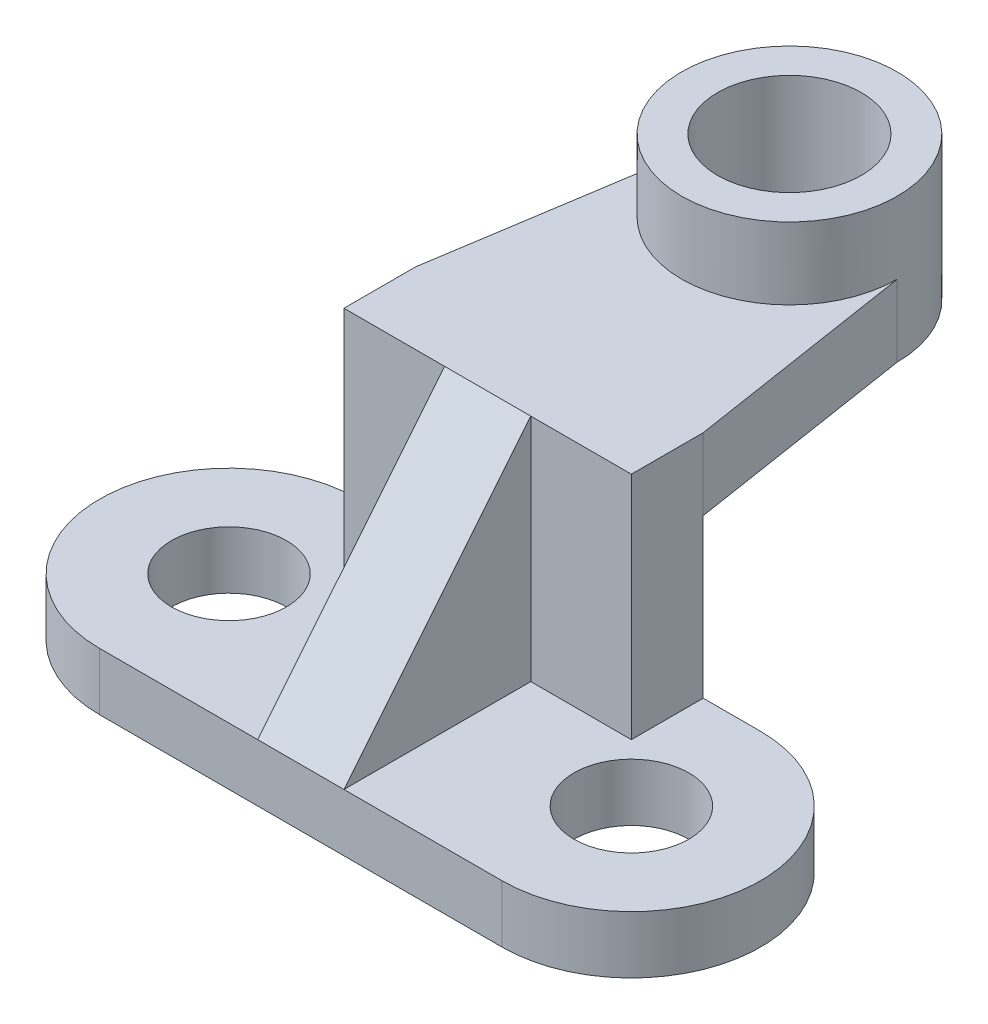
ISO-10303-21;
HEADER;
FILE_DESCRIPTION(('STEP AP214'),'2;1');
FILE_NAME('part.step','',(''),(''),'','','');
FILE_SCHEMA(('AUTOMOTIVE_DESIGN { 1 0 10303 214 1 1 1 1 }'));
ENDSEC;
DATA;
#1=APPLICATION_CONTEXT('core data for automotive mechanical design processes');
#2=APPLICATION_PROTOCOL_DEFINITION('international standard','automotive_design',2000,#1);
#3=PRODUCT_CONTEXT('',#1,'mechanical');
#4=PRODUCT('Part','Part','',(#3));
#5=PRODUCT_RELATED_PRODUCT_CATEGORY('part','',(#4));
#6=PRODUCT_DEFINITION_FORMATION('','',#4);
#7=PRODUCT_DEFINITION_CONTEXT('part definition',#1,'design');
#8=PRODUCT_DEFINITION('design','',#6,#7);
#9=PRODUCT_DEFINITION_SHAPE('','',#8);
#10=(LENGTH_UNIT() NAMED_UNIT(*) SI_UNIT(.MILLI.,.METRE.));
#11=(NAMED_UNIT(*) PLANE_ANGLE_UNIT() SI_UNIT($,.RADIAN.));
#12=(NAMED_UNIT(*) SI_UNIT($,.STERADIAN.) SOLID_ANGLE_UNIT());
#13=UNCERTAINTY_MEASURE_WITH_UNIT(LENGTH_MEASURE(1.E-05),#10,'distance_accuracy_value','');
#14=(GEOMETRIC_REPRESENTATION_CONTEXT(3) GLOBAL_UNCERTAINTY_ASSIGNED_CONTEXT((#13)) GLOBAL_UNIT_ASSIGNED_CONTEXT((#10,
#11,#12)) REPRESENTATION_CONTEXT('',''));
#15=CARTESIAN_POINT('',(0.,0.,0.));
#16=DIRECTION('',(0.,0.,1.));
#17=DIRECTION('',(1.,0.,0.));
#18=AXIS2_PLACEMENT_3D('',#15,#16,#17);
#19=CARTESIAN_POINT('',(-46.,8.,-18.));
#20=DIRECTION('',(0.,0.,1.));
#21=DIRECTION('',(1.,0.,0.));
#22=AXIS2_PLACEMENT_3D('',#19,#20,#21);
#23=PLANE('',#22);
#24=DIRECTION('',(1.,0.,0.));
#25=VECTOR('',#24,1.);
#26=CARTESIAN_POINT('',(-20.,30.,-18.));
#27=LINE('',#26,#25);
#28=CARTESIAN_POINT('',(-20.,30.,-18.));
#29=VERTEX_POINT('',#28);
#30=CARTESIAN_POINT('',(20.,30.,-18.));
#31=VERTEX_POINT('',#30);
#32=EDGE_CURVE('E67',#29,#31,#27,.T.);
#33=ORIENTED_EDGE('',*,*,#32,.T.);
#34=DIRECTION('',(0.,-1.,0.));
#35=VECTOR('',#34,1.);
#36=CARTESIAN_POINT('',(20.,8.,-18.));
#37=LINE('',#36,#35);
#38=CARTESIAN_POINT('',(20.,8.,-18.));
#39=VERTEX_POINT('',#38);
#40=EDGE_CURVE('E222',#31,#39,#37,.T.);
#41=ORIENTED_EDGE('',*,*,#40,.T.);
#42=DIRECTION('',(-1.,0.,0.));
#43=VECTOR('',#42,1.);
#44=CARTESIAN_POINT('',(-46.,8.,-18.));
#45=LINE('',#44,#43);
#46=CARTESIAN_POINT('',(28.,8.,-18.));
#47=VERTEX_POINT('',#46);
#48=EDGE_CURVE('E242',#47,#39,#45,.T.);
#49=ORIENTED_EDGE('',*,*,#48,.F.);
#50=DIRECTION('',(0.,-1.,0.));
#51=VECTOR('',#50,1.);
#52=CARTESIAN_POINT('',(28.,8.,-18.));
#53=LINE('',#52,#51);
#54=CARTESIAN_POINT('',(28.,0.,-18.));
#55=VERTEX_POINT('',#54);
#56=EDGE_CURVE('E259',#47,#55,#53,.T.);
#57=ORIENTED_EDGE('',*,*,#56,.T.);
#58=DIRECTION('',(-1.,0.,0.));
#59=VECTOR('',#58,1.);
#60=CARTESIAN_POINT('',(-46.,0.,-18.));
#61=LINE('',#60,#59);
#62=CARTESIAN_POINT('',(-28.,0.,-18.));
#63=VERTEX_POINT('',#62);
#64=EDGE_CURVE('E233',#55,#63,#61,.T.);
#65=ORIENTED_EDGE('',*,*,#64,.T.);
#66=DIRECTION('',(0.,-1.,0.));
#67=VECTOR('',#66,1.);
#68=CARTESIAN_POINT('',(-28.,8.,-18.));
#69=LINE('',#68,#67);
#70=CARTESIAN_POINT('',(-28.,8.,-18.));
#71=VERTEX_POINT('',#70);
#72=EDGE_CURVE('E270',#63,#71,#69,.F.);
#73=ORIENTED_EDGE('',*,*,#72,.T.);
#74=CARTESIAN_POINT('',(-20.,8.,-18.));
#75=VERTEX_POINT('',#74);
#76=EDGE_CURVE('E249',#75,#71,#45,.T.);
#77=ORIENTED_EDGE('',*,*,#76,.F.);
#78=DIRECTION('',(0.,1.,0.));
#79=VECTOR('',#78,1.);
#80=CARTESIAN_POINT('',(-20.,40.,-18.));
#81=LINE('',#80,#79);
#82=EDGE_CURVE('E204',#75,#29,#81,.T.);
#83=ORIENTED_EDGE('',*,*,#82,.T.);
#84=EDGE_LOOP('',(#33,#41,#49,#57,#65,#73,#77,#83));
#85=FACE_BOUND('',#84,.T.);
#86=ADVANCED_FACE('F41',(#85),#23,.F.);
#87=CARTESIAN_POINT('',(0.,8.,0.));
#88=DIRECTION('',(0.,-1.,0.));
#89=DIRECTION('',(0.,0.,-1.));
#90=AXIS2_PLACEMENT_3D('',#87,#88,#89);
#91=PLANE('',#90);
#92=CARTESIAN_POINT('',(28.,8.,0.));
#93=DIRECTION('',(0.,1.,0.));
#94=DIRECTION('',(0.,0.,1.));
#95=AXIS2_PLACEMENT_3D('',#92,#93,#94);
#96=CIRCLE('',#95,8.00000000000001);
#97=CARTESIAN_POINT('',(28.,8.,8.00000000000001));
#98=VERTEX_POINT('',#97);
#99=EDGE_CURVE('E228',#98,#98,#96,.T.);
#100=ORIENTED_EDGE('',*,*,#99,.F.);
#101=EDGE_LOOP('',(#100));
#102=FACE_BOUND('',#101,.T.);
#103=DIRECTION('',(0.,0.,-1.));
#104=VECTOR('',#103,1.);
#105=CARTESIAN_POINT('',(6.,8.,18.));
#106=LINE('',#105,#104);
#107=CARTESIAN_POINT('',(6.,8.,18.));
#108=VERTEX_POINT('',#107);
#109=CARTESIAN_POINT('',(6.,8.,-8.));
#110=VERTEX_POINT('',#109);
#111=EDGE_CURVE('E192',#108,#110,#106,.T.);
#112=ORIENTED_EDGE('',*,*,#111,.F.);
#113=DIRECTION('',(1.,0.,0.));
#114=VECTOR('',#113,1.);
#115=CARTESIAN_POINT('',(-46.,8.,18.));
#116=LINE('',#115,#114);
#117=CARTESIAN_POINT('',(28.,8.,18.));
#118=VERTEX_POINT('',#117);
#119=EDGE_CURVE('E250',#108,#118,#116,.T.);
#120=ORIENTED_EDGE('',*,*,#119,.T.);
#121=CARTESIAN_POINT('',(28.,8.,0.));
#122=DIRECTION('',(0.,-1.,0.));
#123=DIRECTION('',(0.,0.,-1.));
#124=AXIS2_PLACEMENT_3D('',#121,#122,#123);
#125=CIRCLE('',#124,18.);
#126=EDGE_CURVE('E264',#118,#47,#125,.F.);
#127=ORIENTED_EDGE('',*,*,#126,.T.);
#128=ORIENTED_EDGE('',*,*,#48,.T.);
#129=DIRECTION('',(0.,0.,-1.));
#130=VECTOR('',#129,1.);
#131=CARTESIAN_POINT('',(20.,8.,-8.));
#132=LINE('',#131,#130);
#133=CARTESIAN_POINT('',(20.,8.,-8.));
#134=VERTEX_POINT('',#133);
#135=EDGE_CURVE('E230',#134,#39,#132,.T.);
#136=ORIENTED_EDGE('',*,*,#135,.F.);
#137=DIRECTION('',(-1.,0.,0.));
#138=VECTOR('',#137,1.);
#139=CARTESIAN_POINT('',(20.,8.,-8.));
#140=LINE('',#139,#138);
#141=EDGE_CURVE('E216',#134,#110,#140,.T.);
#142=ORIENTED_EDGE('',*,*,#141,.T.);
#143=EDGE_LOOP('',(#112,#120,#127,#128,#136,#142));
#144=FACE_BOUND('',#143,.T.);
#145=ADVANCED_FACE('F291',(#102,#144),#91,.F.);
#146=CARTESIAN_POINT('',(0.,0.,-8.));
#147=DIRECTION('',(0.,0.,-1.));
#148=DIRECTION('',(-1.,0.,0.));
#149=AXIS2_PLACEMENT_3D('',#146,#147,#148);
#150=PLANE('',#149);
#151=DIRECTION('',(0.,1.,0.));
#152=VECTOR('',#151,1.);
#153=CARTESIAN_POINT('',(6.,8.,-8.));
#154=LINE('',#153,#152);
#155=CARTESIAN_POINT('',(6.,40.,-8.));
#156=VERTEX_POINT('',#155);
#157=EDGE_CURVE('E183',#110,#156,#154,.T.);
#158=ORIENTED_EDGE('',*,*,#157,.F.);
#159=ORIENTED_EDGE('',*,*,#141,.F.);
#160=DIRECTION('',(0.,-1.,0.));
#161=VECTOR('',#160,1.);
#162=CARTESIAN_POINT('',(20.,8.,-8.));
#163=LINE('',#162,#161);
#164=CARTESIAN_POINT('',(20.,40.,-8.));
#165=VERTEX_POINT('',#164);
#166=EDGE_CURVE('E213',#165,#134,#163,.T.);
#167=ORIENTED_EDGE('',*,*,#166,.F.);
#168=DIRECTION('',(1.,0.,0.));
#169=VECTOR('',#168,1.);
#170=CARTESIAN_POINT('',(20.,40.,-8.));
#171=LINE('',#170,#169);
#172=EDGE_CURVE('E208',#156,#165,#171,.T.);
#173=ORIENTED_EDGE('',*,*,#172,.F.);
#174=EDGE_LOOP('',(#158,#159,#167,#173));
#175=FACE_BOUND('',#174,.T.);
#176=ADVANCED_FACE('F305',(#175),#150,.F.);
#177=CARTESIAN_POINT('',(-28.,8.,0.));
#178=DIRECTION('',(0.,1.,0.));
#179=DIRECTION('',(0.,0.,1.));
#180=AXIS2_PLACEMENT_3D('',#177,#178,#179);
#181=CIRCLE('',#180,8.);
#182=CARTESIAN_POINT('',(-28.,8.,8.));
#183=VERTEX_POINT('',#182);
#184=EDGE_CURVE('E237',#183,#183,#181,.T.);
#185=ORIENTED_EDGE('',*,*,#184,.F.);
#186=EDGE_LOOP('',(#185));
#187=FACE_BOUND('',#186,.T.);
#188=CARTESIAN_POINT('',(-28.,8.,18.));
#189=VERTEX_POINT('',#188);
#190=CARTESIAN_POINT('',(-6.,8.,18.));
#191=VERTEX_POINT('',#190);
#192=EDGE_CURVE('E246',#189,#191,#116,.T.);
#193=ORIENTED_EDGE('',*,*,#192,.T.);
#194=DIRECTION('',(0.,0.,-1.));
#195=VECTOR('',#194,1.);
#196=CARTESIAN_POINT('',(-6.,8.,18.));
#197=LINE('',#196,#195);
#198=CARTESIAN_POINT('',(-6.,8.,-8.));
#199=VERTEX_POINT('',#198);
#200=EDGE_CURVE('E187',#191,#199,#197,.T.);
#201=ORIENTED_EDGE('',*,*,#200,.T.);
#202=CARTESIAN_POINT('',(-20.,8.,-8.));
#203=VERTEX_POINT('',#202);
#204=EDGE_CURVE('E214',#199,#203,#140,.T.);
#205=ORIENTED_EDGE('',*,*,#204,.T.);
#206=DIRECTION('',(0.,0.,-1.));
#207=VECTOR('',#206,1.);
#208=CARTESIAN_POINT('',(-20.,8.,-8.));
#209=LINE('',#208,#207);
#210=EDGE_CURVE('E224',#203,#75,#209,.T.);
#211=ORIENTED_EDGE('',*,*,#210,.T.);
#212=ORIENTED_EDGE('',*,*,#76,.T.);
#213=CARTESIAN_POINT('',(-28.,8.,0.));
#214=DIRECTION('',(0.,-1.,0.));
#215=DIRECTION('',(0.,0.,-1.));
#216=AXIS2_PLACEMENT_3D('',#213,#214,#215);
#217=CIRCLE('',#216,18.);
#218=EDGE_CURVE('E51',#71,#189,#217,.F.);
#219=ORIENTED_EDGE('',*,*,#218,.T.);
#220=EDGE_LOOP('',(#193,#201,#205,#211,#212,#219));
#221=FACE_BOUND('',#220,.T.);
#222=ADVANCED_FACE('F280',(#187,#221),#91,.F.);
#223=CARTESIAN_POINT('',(-28.,0.,0.));
#224=DIRECTION('',(0.,-1.,0.));
#225=DIRECTION('',(0.,0.,-1.));
#226=AXIS2_PLACEMENT_3D('',#223,#224,#225);
#227=CYLINDRICAL_SURFACE('',#226,18.);
#228=ORIENTED_EDGE('',*,*,#72,.F.);
#229=CARTESIAN_POINT('',(-28.,0.,0.));
#230=DIRECTION('',(0.,-1.,0.));
#231=DIRECTION('',(0.,0.,-1.));
#232=AXIS2_PLACEMENT_3D('',#229,#230,#231);
#233=CIRCLE('',#232,18.);
#234=CARTESIAN_POINT('',(-28.,0.,18.));
#235=VERTEX_POINT('',#234);
#236=EDGE_CURVE('E272',#235,#63,#233,.T.);
#237=ORIENTED_EDGE('',*,*,#236,.F.);
#238=DIRECTION('',(0.,-1.,0.));
#239=VECTOR('',#238,1.);
#240=CARTESIAN_POINT('',(-28.,8.,18.));
#241=LINE('',#240,#239);
#242=EDGE_CURVE('E269',#189,#235,#241,.T.);
#243=ORIENTED_EDGE('',*,*,#242,.F.);
#244=ORIENTED_EDGE('',*,*,#218,.F.);
#245=EDGE_LOOP('',(#228,#237,#243,#244));
#246=FACE_BOUND('',#245,.T.);
#247=ADVANCED_FACE('F42',(#246),#227,.T.);
#248=CARTESIAN_POINT('',(28.,0.,0.));
#249=DIRECTION('',(0.,-1.,0.));
#250=DIRECTION('',(0.,0.,-1.));
#251=AXIS2_PLACEMENT_3D('',#248,#249,#250);
#252=CYLINDRICAL_SURFACE('',#251,18.);
#253=DIRECTION('',(0.,-1.,0.));
#254=VECTOR('',#253,1.);
#255=CARTESIAN_POINT('',(28.,8.,18.));
#256=LINE('',#255,#254);
#257=CARTESIAN_POINT('',(28.,0.,18.));
#258=VERTEX_POINT('',#257);
#259=EDGE_CURVE('E252',#258,#118,#256,.F.);
#260=ORIENTED_EDGE('',*,*,#259,.F.);
#261=CARTESIAN_POINT('',(28.,0.,0.));
#262=DIRECTION('',(0.,-1.,0.));
#263=DIRECTION('',(0.,0.,-1.));
#264=AXIS2_PLACEMENT_3D('',#261,#262,#263);
#265=CIRCLE('',#264,18.);
#266=EDGE_CURVE('E265',#55,#258,#265,.T.);
#267=ORIENTED_EDGE('',*,*,#266,.F.);
#268=ORIENTED_EDGE('',*,*,#56,.F.);
#269=ORIENTED_EDGE('',*,*,#126,.F.);
#270=EDGE_LOOP('',(#260,#267,#268,#269));
#271=FACE_BOUND('',#270,.T.);
#272=ADVANCED_FACE('F349',(#271),#252,.T.);
#273=CARTESIAN_POINT('',(-46.,8.,18.));
#274=DIRECTION('',(0.,0.,-1.));
#275=DIRECTION('',(-1.,0.,0.));
#276=AXIS2_PLACEMENT_3D('',#273,#274,#275);
#277=PLANE('',#276);
#278=ORIENTED_EDGE('',*,*,#192,.F.);
#279=ORIENTED_EDGE('',*,*,#242,.T.);
#280=DIRECTION('',(1.,0.,0.));
#281=VECTOR('',#280,1.);
#282=CARTESIAN_POINT('',(-46.,0.,18.));
#283=LINE('',#282,#281);
#284=EDGE_CURVE('E254',#235,#258,#283,.T.);
#285=ORIENTED_EDGE('',*,*,#284,.T.);
#286=ORIENTED_EDGE('',*,*,#259,.T.);
#287=ORIENTED_EDGE('',*,*,#119,.F.);
#288=DIRECTION('',(-1.,0.,0.));
#289=VECTOR('',#288,1.);
#290=CARTESIAN_POINT('',(6.,8.,18.));
#291=LINE('',#290,#289);
#292=EDGE_CURVE('E194',#108,#191,#291,.T.);
#293=ORIENTED_EDGE('',*,*,#292,.T.);
#294=EDGE_LOOP('',(#278,#279,#285,#286,#287,#293));
#295=FACE_BOUND('',#294,.T.);
#296=ADVANCED_FACE('F282',(#295),#277,.F.);
#297=CARTESIAN_POINT('',(0.,0.,0.));
#298=DIRECTION('',(0.,-1.,0.));
#299=DIRECTION('',(0.,0.,-1.));
#300=AXIS2_PLACEMENT_3D('',#297,#298,#299);
#301=PLANE('',#300);
#302=CARTESIAN_POINT('',(-28.,0.,0.));
#303=DIRECTION('',(0.,1.,0.));
#304=DIRECTION('',(0.,0.,1.));
#305=AXIS2_PLACEMENT_3D('',#302,#303,#304);
#306=CIRCLE('',#305,8.);
#307=CARTESIAN_POINT('',(-28.,0.,8.));
#308=VERTEX_POINT('',#307);
#309=EDGE_CURVE('E235',#308,#308,#306,.T.);
#310=ORIENTED_EDGE('',*,*,#309,.T.);
#311=EDGE_LOOP('',(#310));
#312=FACE_BOUND('',#311,.T.);
#313=CARTESIAN_POINT('',(28.,0.,0.));
#314=DIRECTION('',(0.,1.,0.));
#315=DIRECTION('',(0.,0.,1.));
#316=AXIS2_PLACEMENT_3D('',#313,#314,#315);
#317=CIRCLE('',#316,8.00000000000001);
#318=CARTESIAN_POINT('',(28.,0.,8.00000000000001));
#319=VERTEX_POINT('',#318);
#320=EDGE_CURVE('E239',#319,#319,#317,.T.);
#321=ORIENTED_EDGE('',*,*,#320,.T.);
#322=EDGE_LOOP('',(#321));
#323=FACE_BOUND('',#322,.T.);
#324=ORIENTED_EDGE('',*,*,#284,.F.);
#325=ORIENTED_EDGE('',*,*,#236,.T.);
#326=ORIENTED_EDGE('',*,*,#64,.F.);
#327=ORIENTED_EDGE('',*,*,#266,.T.);
#328=EDGE_LOOP('',(#324,#325,#326,#327));
#329=FACE_BOUND('',#328,.T.);
#330=ADVANCED_FACE('F359',(#312,#323,#329),#301,.T.);
#331=CARTESIAN_POINT('',(28.,0.,0.));
#332=DIRECTION('',(0.,1.,0.));
#333=DIRECTION('',(0.,0.,1.));
#334=AXIS2_PLACEMENT_3D('',#331,#332,#333);
#335=CYLINDRICAL_SURFACE('',#334,8.00000000000001);
#336=ORIENTED_EDGE('',*,*,#320,.F.);
#337=EDGE_LOOP('',(#336));
#338=FACE_BOUND('',#337,.T.);
#339=ORIENTED_EDGE('',*,*,#99,.T.);
#340=EDGE_LOOP('',(#339));
#341=FACE_BOUND('',#340,.T.);
#342=ADVANCED_FACE('F379',(#338,#341),#335,.F.);
#343=CARTESIAN_POINT('',(-28.,0.,0.));
#344=DIRECTION('',(0.,1.,0.));
#345=DIRECTION('',(0.,0.,1.));
#346=AXIS2_PLACEMENT_3D('',#343,#344,#345);
#347=CYLINDRICAL_SURFACE('',#346,8.);
#348=ORIENTED_EDGE('',*,*,#309,.F.);
#349=EDGE_LOOP('',(#348));
#350=FACE_BOUND('',#349,.T.);
#351=ORIENTED_EDGE('',*,*,#184,.T.);
#352=EDGE_LOOP('',(#351));
#353=FACE_BOUND('',#352,.T.);
#354=ADVANCED_FACE('F373',(#350,#353),#347,.F.);
#355=CARTESIAN_POINT('',(-20.,40.,-8.));
#356=DIRECTION('',(-1.,0.,0.));
#357=DIRECTION('',(0.,0.,1.));
#358=AXIS2_PLACEMENT_3D('',#355,#356,#357);
#359=PLANE('',#358);
#360=ORIENTED_EDGE('',*,*,#82,.F.);
#361=ORIENTED_EDGE('',*,*,#210,.F.);
#362=DIRECTION('',(0.,1.,0.));
#363=VECTOR('',#362,1.);
#364=CARTESIAN_POINT('',(-20.,40.,-8.));
#365=LINE('',#364,#363);
#366=CARTESIAN_POINT('',(-20.,40.,-8.));
#367=VERTEX_POINT('',#366);
#368=EDGE_CURVE('E202',#203,#367,#365,.T.);
#369=ORIENTED_EDGE('',*,*,#368,.T.);
#370=DIRECTION('',(0.,0.,-1.));
#371=VECTOR('',#370,1.);
#372=CARTESIAN_POINT('',(-20.,40.,-8.));
#373=LINE('',#372,#371);
#374=CARTESIAN_POINT('',(-20.,40.,-18.));
#375=VERTEX_POINT('',#374);
#376=EDGE_CURVE('E218',#367,#375,#373,.T.);
#377=ORIENTED_EDGE('',*,*,#376,.T.);
#378=DIRECTION('',(0.,1.,0.));
#379=VECTOR('',#378,1.);
#380=CARTESIAN_POINT('',(-20.,30.,-18.));
#381=LINE('',#380,#379);
#382=EDGE_CURVE('E56',#29,#375,#381,.T.);
#383=ORIENTED_EDGE('',*,*,#382,.F.);
#384=EDGE_LOOP('',(#360,#361,#369,#377,#383));
#385=FACE_BOUND('',#384,.T.);
#386=ADVANCED_FACE('F311',(#385),#359,.T.);
#387=CARTESIAN_POINT('',(20.,8.,-8.));
#388=DIRECTION('',(1.,0.,0.));
#389=DIRECTION('',(0.,0.,-1.));
#390=AXIS2_PLACEMENT_3D('',#387,#388,#389);
#391=PLANE('',#390);
#392=CARTESIAN_POINT('',(20.,40.,-18.));
#393=VERTEX_POINT('',#392);
#394=EDGE_CURVE('E207',#393,#31,#37,.T.);
#395=ORIENTED_EDGE('',*,*,#394,.F.);
#396=DIRECTION('',(0.,0.,-1.));
#397=VECTOR('',#396,1.);
#398=CARTESIAN_POINT('',(20.,40.,-8.));
#399=LINE('',#398,#397);
#400=EDGE_CURVE('E151',#165,#393,#399,.T.);
#401=ORIENTED_EDGE('',*,*,#400,.F.);
#402=ORIENTED_EDGE('',*,*,#166,.T.);
#403=ORIENTED_EDGE('',*,*,#135,.T.);
#404=ORIENTED_EDGE('',*,*,#40,.F.);
#405=EDGE_LOOP('',(#395,#401,#402,#403,#404));
#406=FACE_BOUND('',#405,.T.);
#407=ADVANCED_FACE('F364',(#406),#391,.T.);
#408=CARTESIAN_POINT('',(20.,40.,-8.));
#409=DIRECTION('',(0.,1.,0.));
#410=DIRECTION('',(0.,0.,1.));
#411=AXIS2_PLACEMENT_3D('',#408,#409,#410);
#412=PLANE('',#411);
#413=CARTESIAN_POINT('',(0.,40.,-50.));
#414=DIRECTION('',(0.,1.,0.));
#415=DIRECTION('',(0.,0.,1.));
#416=AXIS2_PLACEMENT_3D('',#413,#414,#415);
#417=CIRCLE('',#416,15.);
#418=CARTESIAN_POINT('',(-15.,40.,-50.));
#419=VERTEX_POINT('',#418);
#420=CARTESIAN_POINT('',(15.,40.,-50.));
#421=VERTEX_POINT('',#420);
#422=EDGE_CURVE('E11',#419,#421,#417,.T.);
#423=ORIENTED_EDGE('',*,*,#422,.F.);
#424=DIRECTION('',(-0.15437688027361,0.,0.988012033751101));
#425=VECTOR('',#424,1.);
#426=CARTESIAN_POINT('',(-15.,40.,-50.));
#427=LINE('',#426,#425);
#428=EDGE_CURVE('E154',#419,#375,#427,.T.);
#429=ORIENTED_EDGE('',*,*,#428,.T.);
#430=ORIENTED_EDGE('',*,*,#376,.F.);
#431=CARTESIAN_POINT('',(-6.,40.,-8.));
#432=VERTEX_POINT('',#431);
#433=EDGE_CURVE('E209',#367,#432,#171,.T.);
#434=ORIENTED_EDGE('',*,*,#433,.T.);
#435=DIRECTION('',(-1.,0.,0.));
#436=VECTOR('',#435,1.);
#437=CARTESIAN_POINT('',(6.,40.,-8.));
#438=LINE('',#437,#436);
#439=EDGE_CURVE('E205',#156,#432,#438,.T.);
#440=ORIENTED_EDGE('',*,*,#439,.F.);
#441=ORIENTED_EDGE('',*,*,#172,.T.);
#442=ORIENTED_EDGE('',*,*,#400,.T.);
#443=DIRECTION('',(-0.15437688027361,0.,-0.988012033751101));
#444=VECTOR('',#443,1.);
#445=CARTESIAN_POINT('',(15.,40.,-50.));
#446=LINE('',#445,#444);
#447=EDGE_CURVE('E144',#393,#421,#446,.T.);
#448=ORIENTED_EDGE('',*,*,#447,.T.);
#449=EDGE_LOOP('',(#423,#429,#430,#434,#440,#441,#442,#448));
#450=FACE_BOUND('',#449,.T.);
#451=ADVANCED_FACE('F150',(#450),#412,.T.);
#452=ORIENTED_EDGE('',*,*,#204,.F.);
#453=DIRECTION('',(0.,1.,0.));
#454=VECTOR('',#453,1.);
#455=CARTESIAN_POINT('',(-6.,8.,-8.));
#456=LINE('',#455,#454);
#457=EDGE_CURVE('E164',#199,#432,#456,.T.);
#458=ORIENTED_EDGE('',*,*,#457,.T.);
#459=ORIENTED_EDGE('',*,*,#433,.F.);
#460=ORIENTED_EDGE('',*,*,#368,.F.);
#461=EDGE_LOOP('',(#452,#458,#459,#460));
#462=FACE_BOUND('',#461,.T.);
#463=ADVANCED_FACE('F309',(#462),#150,.F.);
#464=CARTESIAN_POINT('',(6.,40.,-8.));
#465=DIRECTION('',(0.,-0.630592625094466,-0.776114000116266));
#466=DIRECTION('',(0.,0.776114000116266,-0.630592625094466));
#467=AXIS2_PLACEMENT_3D('',#464,#465,#466);
#468=PLANE('',#467);
#469=DIRECTION('',(0.,-0.776114000116266,0.630592625094466));
#470=VECTOR('',#469,1.);
#471=CARTESIAN_POINT('',(-6.,40.,-8.));
#472=LINE('',#471,#470);
#473=EDGE_CURVE('E198',#432,#191,#472,.T.);
#474=ORIENTED_EDGE('',*,*,#473,.T.);
#475=ORIENTED_EDGE('',*,*,#292,.F.);
#476=DIRECTION('',(0.,-0.776114000116266,0.630592625094466));
#477=VECTOR('',#476,1.);
#478=CARTESIAN_POINT('',(6.,40.,-8.));
#479=LINE('',#478,#477);
#480=EDGE_CURVE('E186',#156,#108,#479,.T.);
#481=ORIENTED_EDGE('',*,*,#480,.F.);
#482=ORIENTED_EDGE('',*,*,#439,.T.);
#483=EDGE_LOOP('',(#474,#475,#481,#482));
#484=FACE_BOUND('',#483,.T.);
#485=ADVANCED_FACE('F286',(#484),#468,.F.);
#486=CARTESIAN_POINT('',(6.,0.,0.));
#487=DIRECTION('',(-1.,0.,0.));
#488=DIRECTION('',(0.,0.,1.));
#489=AXIS2_PLACEMENT_3D('',#486,#487,#488);
#490=PLANE('',#489);
#491=ORIENTED_EDGE('',*,*,#157,.T.);
#492=ORIENTED_EDGE('',*,*,#480,.T.);
#493=ORIENTED_EDGE('',*,*,#111,.T.);
#494=EDGE_LOOP('',(#491,#492,#493));
#495=FACE_BOUND('',#494,.T.);
#496=ADVANCED_FACE('F297',(#495),#490,.F.);
#497=CARTESIAN_POINT('',(-6.,0.,0.));
#498=DIRECTION('',(-1.,0.,0.));
#499=DIRECTION('',(0.,0.,1.));
#500=AXIS2_PLACEMENT_3D('',#497,#498,#499);
#501=PLANE('',#500);
#502=ORIENTED_EDGE('',*,*,#457,.F.);
#503=ORIENTED_EDGE('',*,*,#200,.F.);
#504=ORIENTED_EDGE('',*,*,#473,.F.);
#505=EDGE_LOOP('',(#502,#503,#504));
#506=FACE_BOUND('',#505,.T.);
#507=ADVANCED_FACE('F307',(#506),#501,.T.);
#508=CARTESIAN_POINT('',(0.,30.,-50.));
#509=DIRECTION('',(0.,1.,0.));
#510=DIRECTION('',(0.,0.,1.));
#511=AXIS2_PLACEMENT_3D('',#508,#509,#510);
#512=CYLINDRICAL_SURFACE('',#511,15.);
#513=DIRECTION('',(0.,1.,0.));
#514=VECTOR('',#513,1.);
#515=CARTESIAN_POINT('',(-15.,30.,-50.));
#516=LINE('',#515,#514);
#517=CARTESIAN_POINT('',(-15.,30.,-50.));
#518=VERTEX_POINT('',#517);
#519=EDGE_CURVE('E166',#518,#419,#516,.T.);
#520=ORIENTED_EDGE('',*,*,#519,.T.);
#521=ORIENTED_EDGE('',*,*,#422,.T.);
#522=DIRECTION('',(0.,1.,0.));
#523=VECTOR('',#522,1.);
#524=CARTESIAN_POINT('',(15.,30.,-50.));
#525=LINE('',#524,#523);
#526=CARTESIAN_POINT('',(15.,30.,-50.));
#527=VERTEX_POINT('',#526);
#528=EDGE_CURVE('E158',#527,#421,#525,.T.);
#529=ORIENTED_EDGE('',*,*,#528,.F.);
#530=CARTESIAN_POINT('',(0.,30.,-50.));
#531=DIRECTION('',(0.,1.,0.));
#532=DIRECTION('',(0.,0.,1.));
#533=AXIS2_PLACEMENT_3D('',#530,#531,#532);
#534=CIRCLE('',#533,15.);
#535=EDGE_CURVE('E152',#527,#518,#534,.T.);
#536=ORIENTED_EDGE('',*,*,#535,.T.);
#537=EDGE_LOOP('',(#520,#521,#529,#536));
#538=FACE_BOUND('',#537,.T.);
#539=CARTESIAN_POINT('',(0.,50.,-50.));
#540=DIRECTION('',(0.,1.,0.));
#541=DIRECTION('',(0.,0.,1.));
#542=AXIS2_PLACEMENT_3D('',#539,#540,#541);
#543=CIRCLE('',#542,15.);
#544=CARTESIAN_POINT('',(0.,50.,-35.));
#545=VERTEX_POINT('',#544);
#546=EDGE_CURVE('E177',#545,#545,#543,.T.);
#547=ORIENTED_EDGE('',*,*,#546,.F.);
#548=EDGE_LOOP('',(#547));
#549=FACE_BOUND('',#548,.T.);
#550=ADVANCED_FACE('F170',(#538,#549),#512,.T.);
#551=CARTESIAN_POINT('',(15.,30.,-50.));
#552=DIRECTION('',(0.988012033751101,0.,-0.15437688027361));
#553=DIRECTION('',(-0.15437688027361,0.,-0.988012033751101));
#554=AXIS2_PLACEMENT_3D('',#551,#552,#553);
#555=PLANE('',#554);
#556=ORIENTED_EDGE('',*,*,#447,.F.);
#557=ORIENTED_EDGE('',*,*,#394,.T.);
#558=DIRECTION('',(-0.15437688027361,0.,-0.988012033751101));
#559=VECTOR('',#558,1.);
#560=CARTESIAN_POINT('',(15.,30.,-50.));
#561=LINE('',#560,#559);
#562=EDGE_CURVE('E161',#31,#527,#561,.T.);
#563=ORIENTED_EDGE('',*,*,#562,.T.);
#564=ORIENTED_EDGE('',*,*,#528,.T.);
#565=EDGE_LOOP('',(#556,#557,#563,#564));
#566=FACE_BOUND('',#565,.T.);
#567=ADVANCED_FACE('F157',(#566),#555,.T.);
#568=CARTESIAN_POINT('',(-15.,30.,-50.));
#569=DIRECTION('',(-0.988012033751101,0.,-0.15437688027361));
#570=DIRECTION('',(-0.15437688027361,0.,0.988012033751101));
#571=AXIS2_PLACEMENT_3D('',#568,#569,#570);
#572=PLANE('',#571);
#573=ORIENTED_EDGE('',*,*,#428,.F.);
#574=ORIENTED_EDGE('',*,*,#519,.F.);
#575=DIRECTION('',(-0.15437688027361,0.,0.988012033751101));
#576=VECTOR('',#575,1.);
#577=CARTESIAN_POINT('',(-15.,30.,-50.));
#578=LINE('',#577,#576);
#579=EDGE_CURVE('E316',#518,#29,#578,.T.);
#580=ORIENTED_EDGE('',*,*,#579,.T.);
#581=ORIENTED_EDGE('',*,*,#382,.T.);
#582=EDGE_LOOP('',(#573,#574,#580,#581));
#583=FACE_BOUND('',#582,.T.);
#584=ADVANCED_FACE('F174',(#583),#572,.T.);
#585=CARTESIAN_POINT('',(0.,30.,-50.));
#586=DIRECTION('',(0.,1.,0.));
#587=DIRECTION('',(0.,0.,1.));
#588=AXIS2_PLACEMENT_3D('',#585,#586,#587);
#589=PLANE('',#588);
#590=CARTESIAN_POINT('',(0.,30.,-50.));
#591=DIRECTION('',(0.,1.,0.));
#592=DIRECTION('',(0.,0.,1.));
#593=AXIS2_PLACEMENT_3D('',#590,#591,#592);
#594=CIRCLE('',#593,10.);
#595=CARTESIAN_POINT('',(0.,30.,-40.));
#596=VERTEX_POINT('',#595);
#597=EDGE_CURVE('E46',#596,#596,#594,.T.);
#598=ORIENTED_EDGE('',*,*,#597,.T.);
#599=EDGE_LOOP('',(#598));
#600=FACE_BOUND('',#599,.T.);
#601=ORIENTED_EDGE('',*,*,#535,.F.);
#602=ORIENTED_EDGE('',*,*,#562,.F.);
#603=ORIENTED_EDGE('',*,*,#32,.F.);
#604=ORIENTED_EDGE('',*,*,#579,.F.);
#605=EDGE_LOOP('',(#601,#602,#603,#604));
#606=FACE_BOUND('',#605,.T.);
#607=ADVANCED_FACE('F312',(#600,#606),#589,.F.);
#608=CARTESIAN_POINT('',(0.,50.,-50.));
#609=DIRECTION('',(0.,1.,0.));
#610=DIRECTION('',(0.,0.,1.));
#611=AXIS2_PLACEMENT_3D('',#608,#609,#610);
#612=PLANE('',#611);
#613=ORIENTED_EDGE('',*,*,#546,.T.);
#614=EDGE_LOOP('',(#613));
#615=FACE_BOUND('',#614,.T.);
#616=CARTESIAN_POINT('',(0.,50.,-50.));
#617=DIRECTION('',(0.,1.,0.));
#618=DIRECTION('',(0.,0.,1.));
#619=AXIS2_PLACEMENT_3D('',#616,#617,#618);
#620=CIRCLE('',#619,10.);
#621=CARTESIAN_POINT('',(0.,50.,-40.));
#622=VERTEX_POINT('',#621);
#623=EDGE_CURVE('E176',#622,#622,#620,.T.);
#624=ORIENTED_EDGE('',*,*,#623,.F.);
#625=EDGE_LOOP('',(#624));
#626=FACE_BOUND('',#625,.T.);
#627=ADVANCED_FACE('F328',(#615,#626),#612,.T.);
#628=CARTESIAN_POINT('',(0.,50.,-50.));
#629=DIRECTION('',(0.,-1.,0.));
#630=DIRECTION('',(0.,0.,-1.));
#631=AXIS2_PLACEMENT_3D('',#628,#629,#630);
#632=CYLINDRICAL_SURFACE('',#631,10.);
#633=ORIENTED_EDGE('',*,*,#623,.T.);
#634=EDGE_LOOP('',(#633));
#635=FACE_BOUND('',#634,.T.);
#636=ORIENTED_EDGE('',*,*,#597,.F.);
#637=EDGE_LOOP('',(#636));
#638=FACE_BOUND('',#637,.T.);
#639=ADVANCED_FACE('F330',(#635,#638),#632,.F.);
#640=CLOSED_SHELL('',(#86,#145,#176,#222,#247,#272,#296,#330,#342,#354,#386,#407,#451,#463,#485,
#496,#507,#550,#567,#584,#607,#627,#639));
#641=MANIFOLD_SOLID_BREP('B2',#640);
#642=ADVANCED_BREP_SHAPE_REPRESENTATION('',(#18,#641),#14);
#643=SHAPE_DEFINITION_REPRESENTATION(#9,#642);
ENDSEC;
END-ISO-10303-21;
